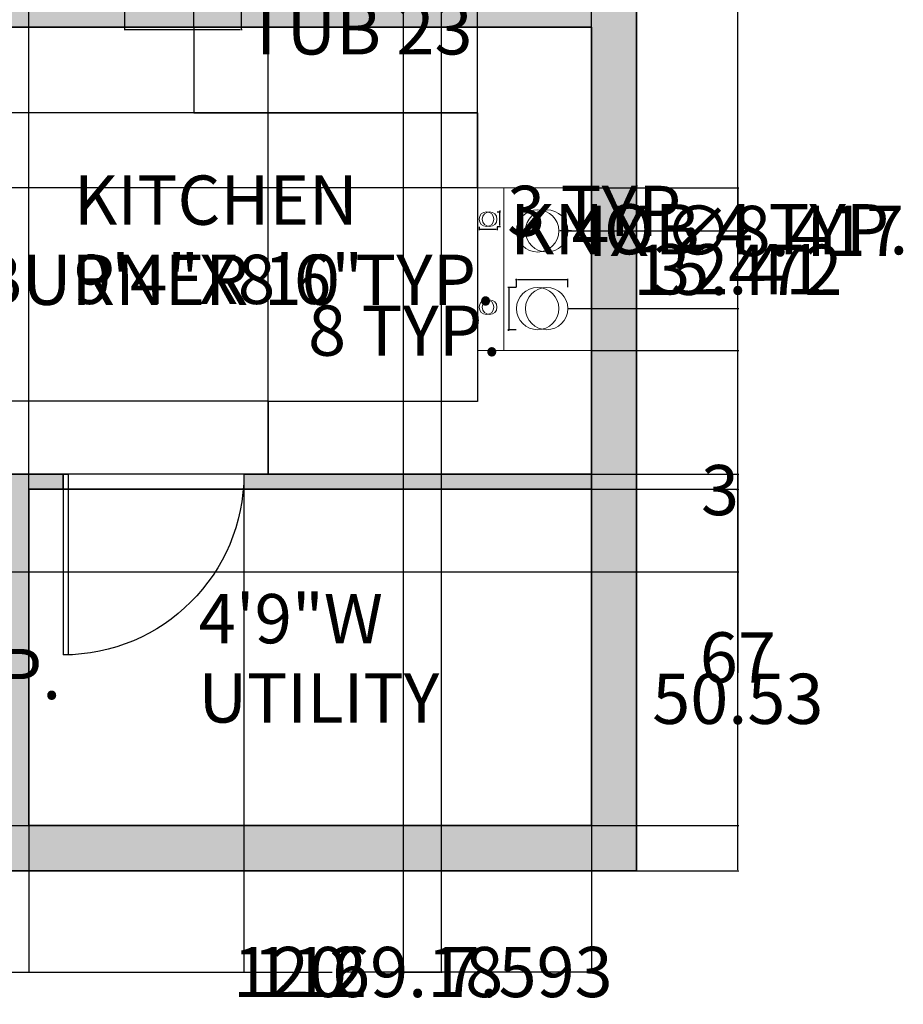
# Model space of a CAD drawing. Units: inches. Extents: x -75 to 484, y -248 to 214.
# Tile 5 of 7: x 291 to 467, y -248 to -52. Entities that reach past the tile are written whole.
import ezdxf

# ---------------------------------------------------------------- set-up
doc = ezdxf.new("R2010")
doc.units = ezdxf.units.IN
doc.header["$MEASUREMENT"] = 0
for name, color, linetype, lineweight in [('A-ANNO-DIMS', 2, 'Continuous', 18), ('A-AREA-IDEN', 7, 'Continuous', 18), ('A-DOOR', 3, 'Continuous', 25), ('A-EQPM', 9, 'Continuous', 18), ('A-FLOR-CASE', 9, 'Continuous', 25), ('A-WALL', 7, 'Continuous', 35)]:
    doc.layers.add(name, color=color, linetype=linetype, lineweight=lineweight)
doc.layers.add('A-WALL-PATT', color=252, linetype='Continuous', lineweight=9, true_color=0x939598)
doc.styles.get("Standard").update_dxf_attribs({"font": 'arial.ttf'})
doc.dimstyles.get("Standard").update_dxf_attribs({"dimtxt": 10, "dimasz": 0.18, "dimexe": 0.18, "dimexo": 0.0625, "dimgap": 0.09, "dimtad": 0, "dimtih": 1, "dimtoh": 1, "dimdec": 0, "dimzin": 0, "dimdsep": 46, "dimlunit": 3, "dimtxsty": 'Standard', "dimcen": 0.09, "dimadec": 0, "dimazin": 0, "dimtfac": 1, "dimtdec": 0, "dimtofl": 0, "dimtmove": 0, "dimatfit": 3, "dimfxl": 1, "dimtolj": 1, "dimtzin": 0, "dimarcsym": 0})

# ---------------------------------------------------------------- blocks, each defined once
blk = doc.blocks.new('DOOR-SINGLE-36')
for p, q in [((35, 36), (35, 0)), ((36, 36), (36, 0))]:
    blk.add_line(p, q)
blk.add_arc((36, 36), 36, 180, 270)
blk = doc.blocks.new('COOKTOP-BURNER')
for centre in [(4.21, 4.21), (6.01, 4.21)]:
    blk.add_circle(centre, 4.21)
blk = doc.blocks.new('COOKTOP-KNOB')
for centre in [(1.47, 1.47), (2.08, 1.47)]:
    blk.add_circle(centre, 1.47)
blk = doc.blocks.new('*D21')
at = {"layer": 'A-ANNO-DIMS', "color": 0, "lineweight": -2, "transparency": 16777216}
for p, q in [((204.49, -180.49), (207.14, -182.4)), ((207, -182.29), (207.1, -182.15)), ((207.1, -182.15), (207.28, -182.15)), ((194.83, -199.19), (206.89, -182.44)), ((192.22, -197.53), (194.87, -199.44))]:
    blk.add_line(p, q, dxfattribs=at)
at = {"layer": 'A-ANNO-DIMS', "color": 0, "transparency": 16777216}
for points in [[(206.87, -182.42), (206.92, -182.46), (207, -182.29)], [(194.8, -199.17), (194.85, -199.2), (194.72, -199.33)]]:
    blk.add_solid(points, dxfattribs=at)
at = {"layer": 'Defpoints', "color": 0, "transparency": 16777216}
for p in [(204.44, -180.45), (207, -182.29), (192.17, -197.49)]:
    blk.add_point(p, dxfattribs=at)
at = {"layer": 'A-ANNO-DIMS', "color": 0, "transparency": 16777216, "insert": (255.32, -182.15), "char_height": 10, "attachment_point": 5}
blk.add_mtext('\\A1;CHAIR 21 TYP.', dxfattribs=at)
blk = doc.blocks.new('*D35')
at = {"layer": 'A-ANNO-DIMS', "color": 0, "lineweight": -2, "transparency": 16777216}
for p, q in [((312.26, -50.35), (312.26, -53.95)), ((335.49, -50.35), (335.49, -53.95)), ((312.44, -53.77), (335.31, -53.77)), ((335.49, -53.77), (335.67, -53.77))]:
    blk.add_line(p, q, dxfattribs=at)
at = {"layer": 'A-ANNO-DIMS', "color": 0, "transparency": 16777216}
for points in [[(312.44, -53.74), (312.44, -53.8), (312.26, -53.77)], [(335.31, -53.74), (335.31, -53.8), (335.49, -53.77)]]:
    blk.add_solid(points, dxfattribs=at)
at = {"layer": 'Defpoints', "color": 0, "transparency": 16777216}
for p in [(312.26, -50.29), (335.49, -50.29), (335.49, -53.77)]:
    blk.add_point(p, dxfattribs=at)
at = {"layer": 'A-ANNO-DIMS', "color": 0, "transparency": 16777216, "insert": (358.96, -53.77), "char_height": 10, "attachment_point": 5}
blk.add_mtext('\\A1;TUB 23', dxfattribs=at)
blk = doc.blocks.new('*D37')
at = {"layer": 'A-ANNO-DIMS', "color": 0, "lineweight": -2, "transparency": 16777216}
for p, q in [((390.31, -103.63), (390.13, -103.63)), ((390.31, -105.1), (390.31, -103.45)), ((400.34, -103.63), (390.49, -103.63)), ((400.52, -105.1), (400.52, -103.45))]:
    blk.add_line(p, q, dxfattribs=at)
at = {"layer": 'A-ANNO-DIMS', "color": 0, "transparency": 16777216}
for points in [[(390.49, -103.6), (390.49, -103.66), (390.31, -103.63)], [(400.34, -103.6), (400.34, -103.66), (400.52, -103.63)]]:
    blk.add_solid(points, dxfattribs=at)
at = {"layer": 'Defpoints', "color": 0, "transparency": 16777216}
for p in [(390.31, -103.63), (390.31, -105.16), (400.52, -105.16)]:
    blk.add_point(p, dxfattribs=at)
at = {"layer": 'A-ANNO-DIMS', "color": 0, "transparency": 16777216, "insert": (334.48, -103.63), "char_height": 10, "attachment_point": 5}
blk.add_mtext('\\A1;BURNER 10 TYP.', dxfattribs=at)
blk = doc.blocks.new('*D38')
at = {"layer": 'A-ANNO-DIMS', "color": 0, "lineweight": -2, "transparency": 16777216}
for p, q in [((390.24, -105.16), (388.59, -105.16)), ((388.77, -105.34), (388.77, -113.4)), ((390.24, -113.58), (388.59, -113.58)), ((388.77, -113.58), (388.77, -113.76)), ((388.77, -113.76), (388.59, -113.76))]:
    blk.add_line(p, q, dxfattribs=at)
at = {"layer": 'A-ANNO-DIMS', "color": 0, "transparency": 16777216}
for points in [[(388.74, -105.34), (388.8, -105.34), (388.77, -105.16)], [(388.74, -113.4), (388.8, -113.4), (388.77, -113.58)]]:
    blk.add_solid(points, dxfattribs=at)
at = {"layer": 'Defpoints', "color": 0, "transparency": 16777216}
for p in [(390.31, -105.16), (388.77, -113.58), (390.31, -113.58)]:
    blk.add_point(p, dxfattribs=at)
at = {"layer": 'A-ANNO-DIMS', "color": 0, "transparency": 16777216, "insert": (368.04, -113.76), "char_height": 10, "attachment_point": 5}
blk.add_mtext('\\A1;8 TYP.', dxfattribs=at)
blk = doc.blocks.new('*D39')
at = {"layer": 'A-ANNO-DIMS', "color": 0, "lineweight": -2, "transparency": 16777216}
for p, q in [((382.86, -93.1), (382.86, -93.75)), ((383.04, -93.57), (386.24, -93.57)), ((386.42, -93.1), (386.42, -93.75)), ((386.42, -93.57), (386.6, -93.57))]:
    blk.add_line(p, q, dxfattribs=at)
at = {"layer": 'A-ANNO-DIMS', "color": 0, "transparency": 16777216}
for points in [[(383.04, -93.54), (383.04, -93.6), (382.86, -93.57)], [(386.24, -93.54), (386.24, -93.6), (386.42, -93.57)]]:
    blk.add_solid(points, dxfattribs=at)
at = {"layer": 'Defpoints', "color": 0, "transparency": 16777216}
for p in [(382.86, -93.04), (386.42, -93.04), (386.42, -93.57)]:
    blk.add_point(p, dxfattribs=at)
at = {"layer": 'A-ANNO-DIMS', "color": 0, "transparency": 16777216, "insert": (428.66, -93.57), "char_height": 10, "attachment_point": 5}
blk.add_mtext('\\A1;KNOB 4 TYP.', dxfattribs=at)
blk = doc.blocks.new('*D40')
at = {"layer": 'A-ANNO-DIMS', "color": 0, "lineweight": -2, "transparency": 16777216}
for p, q in [((386.48, -90.09), (387.13, -90.09)), ((386.95, -90.09), (386.95, -89.91)), ((386.95, -89.91), (387.13, -89.91)), ((386.95, -92.86), (386.95, -90.27)), ((386.48, -93.04), (387.13, -93.04))]:
    blk.add_line(p, q, dxfattribs=at)
at = {"layer": 'A-ANNO-DIMS', "color": 0, "transparency": 16777216}
for points in [[(386.92, -90.27), (386.98, -90.27), (386.95, -90.09)], [(386.92, -92.86), (386.98, -92.86), (386.95, -93.04)]]:
    blk.add_solid(points, dxfattribs=at)
at = {"layer": 'Defpoints', "color": 0, "transparency": 16777216}
for p in [(386.42, -90.09), (386.95, -90.09), (386.42, -93.04)]:
    blk.add_point(p, dxfattribs=at)
at = {"layer": 'A-ANNO-DIMS', "color": 0, "transparency": 16777216, "insert": (407.67, -89.91), "char_height": 10, "attachment_point": 5}
blk.add_mtext('\\A1;3 TYP.', dxfattribs=at)
blk = doc.blocks.new('*D42')
at = {"layer": 'A-ANNO-DIMS', "color": 0, "lineweight": -2, "transparency": 16777216}
for p, q in [((414.27, 147.66), (434.54, 147.66)), ((434.36, 147.48), (434.36, -31.64)), ((434.36, -221.16), (434.36, -42.04)), ((414.27, -221.34), (434.54, -221.34))]:
    blk.add_line(p, q, dxfattribs=at)
at = {"layer": 'A-ANNO-DIMS', "color": 0, "transparency": 16777216}
for points in [[(434.33, 147.48), (434.39, 147.48), (434.36, 147.66)], [(434.33, -221.16), (434.39, -221.16), (434.36, -221.34)]]:
    blk.add_solid(points, dxfattribs=at)
at = {"layer": 'Defpoints', "color": 0, "transparency": 16777216}
for p in [(414.21, 147.66), (414.21, -221.34), (434.36, -221.34)]:
    blk.add_point(p, dxfattribs=at)
at = {"layer": 'A-ANNO-DIMS', "color": 0, "transparency": 16777216, "insert": (434.36, -36.84), "char_height": 10, "attachment_point": 5}
blk.add_mtext('\\A1;369', dxfattribs=at)
blk = doc.blocks.new('*D55')
at = {"layer": 'A-ANNO-DIMS', "color": 0, "lineweight": -2, "transparency": 16777216}
for p, q in [((293.21, -212.41), (293.21, -241.67)), ((405.21, -212.41), (405.21, -241.67)), ((293.39, -241.49), (338.59, -241.49)), ((405.03, -241.49), (359.82, -241.49))]:
    blk.add_line(p, q, dxfattribs=at)
at = {"layer": 'A-ANNO-DIMS', "color": 0, "transparency": 16777216}
for points in [[(293.39, -241.46), (293.39, -241.52), (293.21, -241.49)], [(405.03, -241.46), (405.03, -241.52), (405.21, -241.49)]]:
    blk.add_solid(points, dxfattribs=at)
at = {"layer": 'Defpoints', "color": 0, "transparency": 16777216}
for p in [(293.21, -212.34), (405.21, -212.34), (405.21, -241.49)]:
    blk.add_point(p, dxfattribs=at)
at = {"layer": 'A-ANNO-DIMS', "color": 0, "transparency": 16777216, "insert": (349.21, -241.49), "char_height": 10, "attachment_point": 5}
blk.add_mtext('\\A1;112', dxfattribs=at)
blk = doc.blocks.new('*D57')
at = {"layer": 'A-ANNO-DIMS', "color": 0, "lineweight": -2, "transparency": 16777216}
for p, q in [((285.21, -212.28), (285.21, 167.99)), ((285.39, 167.81), (285.82, 167.81)), ((293.03, 167.81), (292.59, 167.81)), ((293.21, -212.28), (293.21, 167.99))]:
    blk.add_line(p, q, dxfattribs=at)
at = {"layer": 'A-ANNO-DIMS', "color": 0, "transparency": 16777216}
for points in [[(285.39, 167.84), (285.39, 167.78), (285.21, 167.81)], [(293.03, 167.84), (293.03, 167.78), (293.21, 167.81)]]:
    blk.add_solid(points, dxfattribs=at)
at = {"layer": 'Defpoints', "color": 0, "transparency": 16777216}
for p in [(285.21, 167.81), (285.21, -212.34), (293.21, -212.34)]:
    blk.add_point(p, dxfattribs=at)
at = {"layer": 'A-ANNO-DIMS', "color": 0, "transparency": 16777216, "insert": (289.21, 167.81), "char_height": 10, "attachment_point": 5}
blk.add_mtext('\\A1;8', dxfattribs=at)
blk = doc.blocks.new('*D62')
at = {"layer": 'A-ANNO-DIMS', "color": 0, "lineweight": -2, "transparency": 16777216}
for p, q in [((336.03, -142.41), (336.03, -241.67)), ((405.21, -145.41), (405.21, -241.67)), ((336.21, -241.49), (353.62, -241.49)), ((405.03, -241.49), (387.62, -241.49))]:
    blk.add_line(p, q, dxfattribs=at)
at = {"layer": 'A-ANNO-DIMS', "color": 0, "transparency": 16777216}
for points in [[(336.21, -241.46), (336.21, -241.52), (336.03, -241.49)], [(405.03, -241.46), (405.03, -241.52), (405.21, -241.49)]]:
    blk.add_solid(points, dxfattribs=at)
at = {"layer": 'Defpoints', "color": 0, "transparency": 16777216}
for p in [(336.03, -142.34), (405.21, -145.34), (405.21, -241.49)]:
    blk.add_point(p, dxfattribs=at)
at = {"layer": 'A-ANNO-DIMS', "color": 0, "transparency": 16777216, "insert": (370.62, -241.49), "char_height": 10, "attachment_point": 5}
blk.add_mtext('\\A1;69.18', dxfattribs=at)
blk = doc.blocks.new('*D63')
at = {"layer": 'A-ANNO-DIMS', "color": 0, "lineweight": -2, "transparency": 16777216}
for p, q in [((405.27, -145.34), (434.54, -145.34)), ((434.36, -145.52), (434.36, -173.65)), ((434.36, -212.16), (434.36, -184.04)), ((405.27, -212.34), (434.54, -212.34))]:
    blk.add_line(p, q, dxfattribs=at)
at = {"layer": 'A-ANNO-DIMS', "color": 0, "transparency": 16777216}
for points in [[(434.33, -145.52), (434.39, -145.52), (434.36, -145.34)], [(434.33, -212.16), (434.39, -212.16), (434.36, -212.34)]]:
    blk.add_solid(points, dxfattribs=at)
at = {"layer": 'Defpoints', "color": 0, "transparency": 16777216}
for p in [(405.21, -145.34), (405.21, -212.34), (434.36, -212.34)]:
    blk.add_point(p, dxfattribs=at)
at = {"layer": 'A-ANNO-DIMS', "color": 0, "transparency": 16777216, "insert": (434.36, -178.84), "char_height": 10, "attachment_point": 5}
blk.add_mtext('\\A1;67', dxfattribs=at)
blk = doc.blocks.new('*D64')
at = {"layer": 'A-ANNO-DIMS', "color": 0, "lineweight": -2, "transparency": 16777216}
for p, q in [((326.06, -53.28), (326.06, 167.99)), ((326.24, 167.81), (348.67, 167.81)), ((405.03, 167.81), (382.59, 167.81)), ((405.21, -53.28), (405.21, 167.99))]:
    blk.add_line(p, q, dxfattribs=at)
at = {"layer": 'A-ANNO-DIMS', "color": 0, "transparency": 16777216}
for points in [[(326.24, 167.84), (326.24, 167.78), (326.06, 167.81)], [(405.03, 167.84), (405.03, 167.78), (405.21, 167.81)]]:
    blk.add_solid(points, dxfattribs=at)
at = {"layer": 'Defpoints', "color": 0, "transparency": 16777216}
for p in [(405.21, 167.81), (326.06, -53.34), (405.21, -53.34)]:
    blk.add_point(p, dxfattribs=at)
at = {"layer": 'A-ANNO-DIMS', "color": 0, "transparency": 16777216, "insert": (365.63, 167.81), "char_height": 10, "attachment_point": 5}
blk.add_mtext('\\A1;79.15', dxfattribs=at)
blk = doc.blocks.new('*D65')
at = {"layer": 'A-ANNO-DIMS', "color": 0, "lineweight": -2, "transparency": 16777216}
for p, q in [((340.87, -142.28), (340.87, 167.99)), ((341.05, 167.81), (356.07, 167.81)), ((405.03, 167.81), (390.01, 167.81)), ((405.21, -142.28), (405.21, 167.99))]:
    blk.add_line(p, q, dxfattribs=at)
at = {"layer": 'A-ANNO-DIMS', "color": 0, "transparency": 16777216}
for points in [[(341.05, 167.84), (341.05, 167.78), (340.87, 167.81)], [(405.03, 167.84), (405.03, 167.78), (405.21, 167.81)]]:
    blk.add_solid(points, dxfattribs=at)
at = {"layer": 'Defpoints', "color": 0, "transparency": 16777216}
for p in [(405.21, 167.81), (340.87, -142.34), (405.21, -142.34)]:
    blk.add_point(p, dxfattribs=at)
at = {"layer": 'A-ANNO-DIMS', "color": 0, "transparency": 16777216, "insert": (373.04, 167.81), "char_height": 10, "attachment_point": 5}
blk.add_mtext('\\A1;64.34', dxfattribs=at)
blk = doc.blocks.new('*D66')
at = {"layer": 'A-ANNO-DIMS', "color": 0, "lineweight": -2, "transparency": 16777216}
for p, q in [((382.57, -85.27), (382.57, 167.99)), ((382.75, 167.81), (405.03, 167.81)), ((405.21, -85.27), (405.21, 167.99)), ((405.21, 167.81), (405.39, 167.81))]:
    blk.add_line(p, q, dxfattribs=at)
at = {"layer": 'A-ANNO-DIMS', "color": 0, "transparency": 16777216}
for points in [[(382.75, 167.84), (382.75, 167.78), (382.57, 167.81)], [(405.03, 167.84), (405.03, 167.78), (405.21, 167.81)]]:
    blk.add_solid(points, dxfattribs=at)
at = {"layer": 'Defpoints', "color": 0, "transparency": 16777216}
for p in [(405.21, 167.81), (382.57, -85.33), (405.21, -85.33)]:
    blk.add_point(p, dxfattribs=at)
at = {"layer": 'A-ANNO-DIMS', "color": 0, "transparency": 16777216, "insert": (426.32, 167.81), "char_height": 10, "attachment_point": 5}
blk.add_mtext('\\A1;22.643', dxfattribs=at)
blk = doc.blocks.new('*D67')
at = {"layer": 'A-ANNO-DIMS', "color": 0, "lineweight": -2, "transparency": 16777216}
for p, q in [((325.99, -53.34), (-5.12, -53.34)), ((-4.94, -53.52), (-4.94, -56.68)), ((-4.94, -70.23), (-4.94, -67.07)), ((325.99, -70.41), (-5.12, -70.41))]:
    blk.add_line(p, q, dxfattribs=at)
at = {"layer": 'A-ANNO-DIMS', "color": 0, "transparency": 16777216}
for points in [[(-4.97, -53.52), (-4.91, -53.52), (-4.94, -53.34)], [(-4.97, -70.23), (-4.91, -70.23), (-4.94, -70.41)]]:
    blk.add_solid(points, dxfattribs=at)
at = {"layer": 'Defpoints', "color": 0, "transparency": 16777216}
for p in [(326.06, -53.34), (-4.94, -70.41), (326.06, -70.41)]:
    blk.add_point(p, dxfattribs=at)
at = {"layer": 'A-ANNO-DIMS', "color": 0, "transparency": 16777216, "insert": (-4.94, -61.88), "char_height": 10, "attachment_point": 5}
blk.add_mtext('\\A1;17.068', dxfattribs=at)
blk = doc.blocks.new('*D68')
at = {"layer": 'A-ANNO-DIMS', "color": 0, "lineweight": -2, "transparency": 16777216}
for p, q in [((340.8, -127.84), (-5.12, -127.84)), ((-4.94, -128.02), (-4.94, -129.9)), ((-4.94, -142.16), (-4.94, -140.29)), ((340.8, -142.34), (-5.12, -142.34))]:
    blk.add_line(p, q, dxfattribs=at)
at = {"layer": 'A-ANNO-DIMS', "color": 0, "transparency": 16777216}
for points in [[(-4.97, -128.02), (-4.91, -128.02), (-4.94, -127.84)], [(-4.97, -142.16), (-4.91, -142.16), (-4.94, -142.34)]]:
    blk.add_solid(points, dxfattribs=at)
at = {"layer": 'Defpoints', "color": 0, "transparency": 16777216}
for p in [(340.87, -127.84), (-4.94, -142.34), (340.87, -142.34)]:
    blk.add_point(p, dxfattribs=at)
at = {"layer": 'A-ANNO-DIMS', "color": 0, "transparency": 16777216, "insert": (-4.94, -135.09), "char_height": 10, "attachment_point": 5}
blk.add_mtext('\\A1;14.5', dxfattribs=at)
blk = doc.blocks.new('*D70')
at = {"layer": 'A-ANNO-DIMS', "color": 0, "lineweight": -2, "transparency": 16777216}
for p, q in [((285.21, -53.41), (285.21, -241.67)), ((405.21, -53.41), (405.21, -241.67)), ((285.39, -241.49), (334.56, -241.49)), ((405.03, -241.49), (355.86, -241.49))]:
    blk.add_line(p, q, dxfattribs=at)
at = {"layer": 'A-ANNO-DIMS', "color": 0, "transparency": 16777216}
for points in [[(285.39, -241.46), (285.39, -241.52), (285.21, -241.49)], [(405.03, -241.46), (405.03, -241.52), (405.21, -241.49)]]:
    blk.add_solid(points, dxfattribs=at)
at = {"layer": 'Defpoints', "color": 0, "transparency": 16777216}
for p in [(285.21, -53.34), (405.21, -53.34), (405.21, -241.49)]:
    blk.add_point(p, dxfattribs=at)
at = {"layer": 'A-ANNO-DIMS', "color": 0, "transparency": 16777216, "insert": (345.21, -241.49), "char_height": 10, "attachment_point": 5}
blk.add_mtext('\\A1;120', dxfattribs=at)
blk = doc.blocks.new('*D71')
at = {"layer": 'A-ANNO-DIMS', "color": 0, "lineweight": -2, "transparency": 16777216}
for p, q in [((405.27, -85.33), (434.54, -85.33)), ((434.36, -85.51), (434.36, -96.34)), ((434.36, -117.56), (434.36, -106.74)), ((405.27, -117.74), (434.54, -117.74))]:
    blk.add_line(p, q, dxfattribs=at)
at = {"layer": 'A-ANNO-DIMS', "color": 0, "transparency": 16777216}
for points in [[(434.33, -85.51), (434.39, -85.51), (434.36, -85.33)], [(434.33, -117.56), (434.39, -117.56), (434.36, -117.74)]]:
    blk.add_solid(points, dxfattribs=at)
at = {"layer": 'Defpoints', "color": 0, "transparency": 16777216}
for p in [(405.21, -85.33), (405.21, -117.74), (434.36, -117.74)]:
    blk.add_point(p, dxfattribs=at)
at = {"layer": 'A-ANNO-DIMS', "color": 0, "transparency": 16777216, "insert": (434.36, -101.54), "char_height": 10, "attachment_point": 5}
blk.add_mtext('\\A1;32.41', dxfattribs=at)
blk = doc.blocks.new('*D72')
at = {"layer": 'A-ANNO-DIMS', "color": 0, "lineweight": -2, "transparency": 16777216}
for p, q in [((382.5, -70.41), (-5.12, -70.41)), ((-4.94, -70.59), (-4.94, -72.68)), ((-4.94, -85.15), (-4.94, -83.07)), ((382.5, -85.33), (-5.12, -85.33))]:
    blk.add_line(p, q, dxfattribs=at)
at = {"layer": 'A-ANNO-DIMS', "color": 0, "transparency": 16777216}
for points in [[(-4.97, -70.59), (-4.91, -70.59), (-4.94, -70.41)], [(-4.97, -85.15), (-4.91, -85.15), (-4.94, -85.33)]]:
    blk.add_solid(points, dxfattribs=at)
at = {"layer": 'Defpoints', "color": 0, "transparency": 16777216}
for p in [(382.57, -70.41), (-4.94, -85.33), (382.57, -85.33)]:
    blk.add_point(p, dxfattribs=at)
at = {"layer": 'A-ANNO-DIMS', "color": 0, "transparency": 16777216, "insert": (-4.94, -77.87), "char_height": 10, "attachment_point": 5}
blk.add_mtext('\\A1;14.92', dxfattribs=at)
blk = doc.blocks.new('*D73')
at = {"layer": 'A-ANNO-DIMS', "color": 0, "lineweight": -2, "transparency": 16777216}
for p, q in [((405.27, -142.34), (434.54, -142.34)), ((434.36, -142.52), (434.36, -145.16)), ((405.27, -145.34), (434.54, -145.34)), ((434.36, -145.52), (434.18, -145.52)), ((434.36, -145.34), (434.36, -145.52))]:
    blk.add_line(p, q, dxfattribs=at)
at = {"layer": 'A-ANNO-DIMS', "color": 0, "transparency": 16777216}
for points in [[(434.33, -142.52), (434.39, -142.52), (434.36, -142.34)], [(434.33, -145.16), (434.39, -145.16), (434.36, -145.34)]]:
    blk.add_solid(points, dxfattribs=at)
at = {"layer": 'Defpoints', "color": 0, "transparency": 16777216}
for p in [(405.21, -142.34), (405.21, -145.34), (434.36, -145.34)]:
    blk.add_point(p, dxfattribs=at)
at = {"layer": 'A-ANNO-DIMS', "color": 0, "transparency": 16777216, "insert": (430.82, -145.52), "char_height": 10, "attachment_point": 5}
blk.add_mtext('\\A1;3', dxfattribs=at)
blk = doc.blocks.new('*D74')
at = {"layer": 'A-ANNO-DIMS', "color": 0, "lineweight": -2, "transparency": 16777216}
for p, q in [((24.27, -161.82), (434.54, -161.82)), ((434.36, -162), (434.36, -181.88)), ((434.36, -212.16), (434.36, -192.28)), ((24.27, -212.34), (434.54, -212.34))]:
    blk.add_line(p, q, dxfattribs=at)
at = {"layer": 'A-ANNO-DIMS', "color": 0, "transparency": 16777216}
for points in [[(434.33, -162), (434.39, -162), (434.36, -161.82)], [(434.33, -212.16), (434.39, -212.16), (434.36, -212.34)]]:
    blk.add_solid(points, dxfattribs=at)
at = {"layer": 'Defpoints', "color": 0, "transparency": 16777216}
for p in [(24.21, -161.82), (434.36, -161.82), (24.21, -212.34)]:
    blk.add_point(p, dxfattribs=at)
at = {"layer": 'A-ANNO-DIMS', "color": 0, "transparency": 16777216, "insert": (434.36, -187.08), "char_height": 10, "attachment_point": 5}
blk.add_mtext('\\A1;50.53', dxfattribs=at)
blk = doc.blocks.new('*D80')
at = {"layer": 'A-ANNO-DIMS', "color": 0, "lineweight": -2, "transparency": 16777216}
for p, q in [((367.71, -42.41), (367.71, -241.67)), ((375.3, -50.41), (375.3, -241.67)), ((367.89, -241.49), (375.12, -241.49)), ((375.3, -241.49), (375.48, -241.49))]:
    blk.add_line(p, q, dxfattribs=at)
at = {"layer": 'A-ANNO-DIMS', "color": 0, "transparency": 16777216}
for points in [[(367.89, -241.46), (367.89, -241.52), (367.71, -241.49)], [(375.12, -241.46), (375.12, -241.52), (375.3, -241.49)]]:
    blk.add_solid(points, dxfattribs=at)
at = {"layer": 'Defpoints', "color": 0, "transparency": 16777216}
for p in [(367.71, -42.34), (375.3, -50.34), (375.3, -241.49)]:
    blk.add_point(p, dxfattribs=at)
at = {"layer": 'A-ANNO-DIMS', "color": 0, "transparency": 16777216, "insert": (392.4, -241.49), "char_height": 10, "attachment_point": 5}
blk.add_mtext('\\A1;7.593', dxfattribs=at)
blk = doc.blocks.new('*D82')
at = {"layer": 'A-ANNO-DIMS', "color": 0, "lineweight": -2, "transparency": 16777216}
for p, q in [((400.59, -93.9), (434.54, -93.9)), ((434.36, -94.08), (434.36, -96.44)), ((434.36, -109.19), (434.36, -106.83)), ((400.59, -109.37), (434.54, -109.37))]:
    blk.add_line(p, q, dxfattribs=at)
at = {"layer": 'A-ANNO-DIMS', "color": 0, "transparency": 16777216}
for points in [[(434.33, -94.08), (434.39, -94.08), (434.36, -93.9)], [(434.33, -109.19), (434.39, -109.19), (434.36, -109.37)]]:
    blk.add_solid(points, dxfattribs=at)
at = {"layer": 'Defpoints', "color": 0, "transparency": 16777216}
for p in [(400.52, -93.9), (400.52, -109.37), (434.36, -109.37)]:
    blk.add_point(p, dxfattribs=at)
at = {"layer": 'A-ANNO-DIMS', "color": 0, "transparency": 16777216, "insert": (434.36, -101.64), "char_height": 10, "attachment_point": 5}
blk.add_mtext('\\A1;15.472', dxfattribs=at)
blk = doc.blocks.new('*D88')
at = {"layer": 'A-ANNO-DIMS', "color": 0, "lineweight": -2, "transparency": 16777216}
for p, q in [((394.42, -93.9), (394.6, -93.9)), ((394.51, -93.99), (394.51, -93.81)), ((401.25, -93.9), (398.9, -93.9))]:
    blk.add_line(p, q, dxfattribs=at)
at = {"layer": 'A-ANNO-DIMS', "color": 0, "transparency": 16777216}
blk.add_solid([(398.9, -93.87), (398.9, -93.93), (398.72, -93.9)], dxfattribs=at)
at = {"layer": 'Defpoints', "color": 0, "transparency": 16777216}
for p in [(390.31, -93.9), (398.72, -93.9)]:
    blk.add_point(p, dxfattribs=at)
at = {"layer": 'A-ANNO-DIMS', "color": 0, "transparency": 16777216, "insert": (434.33, -93.9), "char_height": 10, "attachment_point": 5}
blk.add_mtext('\\A1;4X ∅8.417', dxfattribs=at)

msp = doc.modelspace()

# ---------------------------------------------------------------- hatches: boundary and pattern name
at = {"layer": 'A-WALL-PATT'}
h = msp.add_hatch(color=256, dxfattribs=at)
h.dxf.hatch_style = 1
h.paths.add_polyline_path([(184.9004, 147.6567), (15.2094, 147.6567), (15.2094, 92.5031), (24.2094, 92.5031), (24.2094, 138.6567), (186.0436, 138.6567, -0.06325422)])
h.paths.add_polyline_path([(414.2094, 147.6567), (249.2094, 147.6567), (220.9004, 147.6567), (220.9004, 138.6567), (240.2094, 138.6567), (240.2094, 18.6567), (240.2094, 9.6567), (249.2094, 9.6567), (249.2094, 45.6567), (249.2094, 138.6567), (405.2094, 138.6567), (405.2094, 98.3029), (414.2094, 98.3029)])
h.paths.add_polyline_path([(159.2094, 18.6567), (24.2094, 18.6567), (24.2094, 44.5861), (15.2094, 44.5861), (15.2094, 9.6567), (15.2094, -3.1791), (24.2094, -3.1791), (24.2094, 9.6567), (132.2094, 9.6567), (132.2094, -50.3433), (83.7394, -50.3433), (83.7394, -53.3433), (132.2094, -53.3433), (159.2094, -53.3433), (159.2094, -50.3433), (135.2094, -50.3433), (135.2094, 9.6567), (159.2094, 9.6567)])
h.paths.add_polyline_path([(53.8898, -50.3433), (24.2094, -50.3433), (24.2094, -27.303), (15.2094, -27.303), (15.2094, -50.3433), (15.2094, -53.3433), (15.2094, -74.0487), (24.2094, -74.0487), (24.2094, -53.3433), (53.7394, -53.3433, -0.02504709)])
h.paths.add_polyline_path([(24.2094, -121.9657), (15.2094, -121.9657), (15.2094, -212.3433), (15.2094, -221.3433), (24.2094, -221.3433), (84.3017, -221.3433), (84.3017, -212.3433), (24.2094, -212.3433)])
h.paths.add_polyline_path([(414.2094, -155.3433), (414.2094, -53.3433), (414.2094, -50.3433), (414.2094, -36.8417), (405.2094, -36.8417), (405.2094, -50.3433), (309.2094, -50.3433), (309.2094, 16.0463), (324.2573, 16.0463), (324.2573, 18.6567), (284.0663, 18.6567, -0.06325422), (285.2094, 9.6567), (306.2094, 9.6567), (306.2094, -50.3433), (285.2094, -50.3433), (285.2094, -53.3433), (309.2094, -53.3433), (405.2094, -53.3433), (405.2094, -212.3433), (293.2094, -212.3433), (293.2094, -158.3433), (293.2094, -145.3433), (300.0339, -145.3433), (300.0339, -142.3433), (285.2094, -142.3433), (159.2094, -142.3433), (159.2094, -89.3433, -0.02086055), (156.2094, -89.218), (156.2094, -212.3433), (131.9001, -212.3433), (131.9001, -221.3433), (156.2094, -221.3433), (165.2094, -221.3433), (285.2094, -221.3433), (288.6713, -221.3433), (293.2094, -221.3433), (405.2094, -221.3433), (414.2094, -221.3433)])
h.paths.add_polyline_path([(165.2094, -212.3433), (165.2094, -151.3433), (285.2094, -151.3433), (285.2094, -212.3433)], flags=16)
h.paths.add_polyline_path([(189.462, -195.5437), (182.159, -190.2838, -0.23606798), (182.5164, -188.0765), (181.7049, -187.4921), (185.5037, -182.2177), (184.648, -181.6013, -0.04492589), (180.0821, -186.3232), (179.2706, -185.7388), (189.206, -171.9443), (190.0174, -172.5287, -0.04492589), (186.9857, -178.3556), (187.8415, -178.9719), (191.6403, -173.6976), (192.4517, -174.282, -0.23606798), (194.432, -173.2435), (201.735, -178.5034, -0.23606798), (201.3776, -180.7107), (202.189, -181.2952, -0.11764706), (192.2537, -195.0897), (191.4423, -194.5053, -0.23606798)], flags=0)
h.paths.add_polyline_path([(253.751, -177.9543), (254.5293, -177.3263, -0.23606798), (254.0517, -175.1419), (261.056, -169.4904, -0.23606798), (263.0902, -170.419), (263.8684, -169.7911), (267.95, -174.8498), (268.7708, -174.1875, -0.04492589), (265.425, -168.5352), (266.2032, -167.9073), (276.8782, -181.1378), (276.0999, -181.7657, -0.04492589), (271.2826, -177.3006), (270.4618, -177.9629), (274.5434, -183.0216), (273.7651, -183.6495, -0.23606798), (274.2427, -185.834), (267.2383, -191.4854, -0.23606798), (265.2042, -190.5568), (264.4259, -191.1848, -0.11764706)], flags=0)
h.paths.add_polyline_path([(405.2094, -142.3433), (336.0339, -142.3433, -0.02086055), (335.9087, -145.3433), (405.2094, -145.3433)], flags=17)
h.paths.add_polyline_path([(414.2094, 50.4831), (405.2094, 50.4831), (405.2094, 18.6567), (354.2573, 18.6567, -0.02178446), (354.1435, 16.0463), (405.2094, 16.0463), (405.2094, -14.6494), (414.2094, -14.6494), (414.2094, 9.6567)])
h.paths.add_polyline_path([(200.2091, -179.9247), (255.2702, -179.9247), (255.2702, -168.0448), (200.2091, -168.0448)], flags=8)
h.paths.add_polyline_path([(200.2352, -167.6036), (249.7883, -167.6036), (249.7883, -155.8804), (200.2352, -155.8804)], flags=8)

# ---------------------------------------------------------------- linework, layer by layer
at = {"layer": 'A-DOOR'}
msp.add_line((300.0339, -142.3433), (301.0339, -142.3433), dxfattribs=at)
at = {"layer": 'A-EQPM'}
msp.add_line((387.7545, -85.3314), (387.7545, -117.7421), dxfattribs=at)
msp.add_lwpolyline([(382.5668, -85.3314), (405.2094, -85.3314), (405.2094, -117.7421), (382.5668, -117.7421)], close=True, dxfattribs=at)
at = {"layer": 'A-FLOR-CASE'}
for p, q in [((326.0553, -53.3433), (326.0553, -70.4114)), ((326.0553, -70.4114), (382.5668, -70.4114)), ((382.5668, -70.4114), (382.5668, -127.8437)), ((382.5668, -127.8437), (340.8661, -127.8437)), ((340.8661, -127.8437), (340.8661, -142.3433))]:
    msp.add_line(p, q, dxfattribs=at)
at = {"layer": 'A-WALL'}
for p, q in [((414.2094, -50.3433), (414.2094, -53.3433)), ((309.2094, -53.3433), (285.2094, -53.3433)), ((405.2094, -53.3433), (309.2094, -53.3433)), ((405.2094, -53.3433), (405.2094, -212.3433)), ((414.2094, -53.3433), (414.2094, -155.3433)), ((301.0339, -142.3433), (285.2094, -142.3433)), ((300.0339, -142.3433), (300.0339, -145.3433)), ((405.2094, -142.3433), (336.0339, -142.3433)), ((293.2094, -212.3433), (293.2094, -145.3433)), ((405.2094, -145.3433), (293.2094, -145.3433)), ((414.2094, -155.3433), (414.2094, -221.3433)), ((293.2094, -212.3433), (293.2094, -158.3433)), ((405.2094, -158.3433), (405.2094, -212.3433)), ((414.2094, -158.3433), (414.2094, -212.3433)), ((405.2094, -212.3433), (293.2094, -212.3433)), ((293.2094, -221.3433), (288.6713, -221.3433)), ((405.2094, -221.3433), (293.2094, -221.3433)), ((414.2094, -221.3433), (405.2094, -221.3433))]:
    msp.add_line(p, q, dxfattribs=at)

# ---------------------------------------------------------------- block references
at = {"layer": 'A-DOOR', "extrusion": (0, 0, -1), "zscale": -1}
msp.add_blockref('DOOR-SINGLE-36', (-336.0339, -178.3433), dxfattribs=at)
at = {"layer": 'A-EQPM'}
for name, p in [('COOKTOP-KNOB', (382.8637, -93.0412)), ('COOKTOP-BURNER', (390.3065, -98.1074)), ('COOKTOP-KNOB', (382.8637, -110.5561))]:
    msp.add_blockref(name, p, dxfattribs=at)
at = {"layer": 'A-EQPM', "rotation": 180}
msp.add_blockref('COOKTOP-BURNER', (400.5232, -105.1627), dxfattribs=at)

# ---------------------------------------------------------------- texts
at = {"layer": 'A-AREA-IDEN'}
for s, p in [('KITCHEN', (302.1992, -92.6869)), ('9\'4"X8\'6"', (302.1992, -108.4628)), ('4\'9"W', (326.9984, -176.032)), ('UTILITY', (326.9984, -191.8079))]:
    msp.add_text(s, height=9.82058, dxfattribs=at).set_placement(p)

# ---------------------------------------------------------------- dimensions: what is measured, and where the dimension line sits
at = {"layer": 'A-ANNO-DIMS'}
for base, p1, p2, override, picture, middle in [((285.2094, 167.8067), (293.2094, -212.3433), (285.2094, -212.3433), {"dimdec": 0, "dimlfac": 1, "dimrnd": 0, "dimzin": 0, "dimdsep": 46, "dimlunit": 2}, '*D57', (289.2094, 167.8067)), ((405.2094, 167.8067), (326.0553, -53.3433), (405.2094, -53.3433), {"dimdec": 2, "dimlfac": 1, "dimrnd": 0, "dimzin": 0, "dimdsep": 46, "dimlunit": 2}, '*D64', (365.6324, 167.8067)), ((405.2094, 167.8067), (340.8661, -142.3433), (405.2094, -142.3433), {"dimdec": 2, "dimlfac": 1, "dimrnd": 0, "dimzin": 0, "dimdsep": 46, "dimlunit": 2}, '*D65', (373.0378, 167.8067)), ((405.2094, 167.8067), (382.5668, -85.3314), (405.2094, -85.3314), {"dimdec": 3, "dimlfac": 1, "dimrnd": 0, "dimzin": 0, "dimdsep": 46, "dimlunit": 2}, '*D66', (426.3218, 167.8067)), ((375.3026, -241.4933), (367.7094, -42.3433), (375.3026, -50.3433), {"dimdec": 3, "dimlfac": 1, "dimrnd": 0, "dimzin": 0, "dimdsep": 46, "dimlunit": 2}, '*D80', (392.4041, -241.4933)), ((405.2094, -241.4933), (285.2094, -53.3433), (405.2094, -53.3433), {"dimdec": 0, "dimlfac": 1, "dimrnd": 0, "dimzin": 0, "dimdsep": 46, "dimlunit": 2}, '*D70', (345.2094, -241.4933)), ((405.2094, -241.4933), (336.0339, -142.3433), (405.2094, -145.3433), {"dimdec": 2, "dimlfac": 1, "dimrnd": 0, "dimzin": 0, "dimdsep": 46, "dimlunit": 2}, '*D62', (370.6216, -241.4933)), ((405.2094, -241.4933), (293.2094, -212.3433), (405.2094, -212.3433), {"dimdec": 0, "dimlfac": 1, "dimrnd": 0, "dimzin": 0, "dimdsep": 46, "dimlunit": 2}, '*D55', (349.2094, -241.4933))]:
    dim = msp.add_linear_dim(base=base, p1=p1, p2=p2, dimstyle='Standard', override=override, dxfattribs=at)
    dim.commit()
    dim.dimension.update_dxf_attribs({"geometry": picture, "text_midpoint": middle})
for base, p1, p2, override, picture, middle in [((434.3594, -221.3433), (414.2094, 147.6567), (414.2094, -221.3433), {"dimdec": 0, "dimlfac": 1, "dimrnd": 0, "dimzin": 0, "dimdsep": 46, "dimlunit": 2}, '*D42', (434.3594, -36.8433)), ((-4.9406, -70.4114), (326.0553, -53.3433), (326.0553, -70.4114), {"dimdec": 3, "dimlfac": 1, "dimrnd": 0, "dimzin": 0, "dimdsep": 46, "dimlunit": 2}, '*D67', (-4.9406, -61.8773)), ((-4.9406, -85.3314), (382.5668, -70.4114), (382.5668, -85.3314), {"dimdec": 2, "dimlfac": 1, "dimrnd": 0, "dimzin": 0, "dimdsep": 46, "dimlunit": 2}, '*D72', (-4.9406, -77.8714)), ((434.3594, -117.7421), (405.2094, -85.3314), (405.2094, -117.7421), {"dimdec": 2, "dimlfac": 1, "dimrnd": 0, "dimzin": 0, "dimdsep": 46, "dimlunit": 2}, '*D71', (434.3594, -101.5367)), ((434.3594, -109.3712), (400.5232, -93.899), (400.5232, -109.3712), {"dimdec": 3, "dimlfac": 1, "dimrnd": 0, "dimzin": 0, "dimdsep": 46, "dimlunit": 2}, '*D82', (434.3594, -101.6351)), ((-4.9406, -142.3433), (340.8661, -127.8437), (340.8661, -142.3433), {"dimdec": 1, "dimlfac": 1, "dimrnd": 0, "dimzin": 0, "dimdsep": 46, "dimlunit": 2}, '*D68', (-4.9406, -135.0935)), ((434.3594, -145.3433), (405.2094, -142.3433), (405.2094, -145.3433), {"dimdec": 0, "dimlfac": 1, "dimrnd": 0, "dimzin": 0, "dimdsep": 46, "dimlunit": 2}, '*D73', (430.8152, -145.5233)), ((434.3594, -212.3433), (405.2094, -145.3433), (405.2094, -212.3433), {"dimdec": 0, "dimlfac": 1, "dimrnd": 0, "dimzin": 0, "dimdsep": 46, "dimlunit": 2}, '*D63', (434.3594, -178.8433)), ((434.3594, -161.8152), (24.2094, -212.3433), (24.2094, -161.8152), {"dimdec": 2, "dimlfac": 1, "dimrnd": 0, "dimzin": 0, "dimdsep": 46, "dimlunit": 2}, '*D74', (434.3594, -187.0792))]:
    dim = msp.add_linear_dim(base=base, p1=p1, p2=p2, angle=90, dimstyle='Standard', override=override, dxfattribs=at)
    dim.commit()
    dim.dimension.update_dxf_attribs({"geometry": picture, "text_midpoint": middle})
for base, p1, p2, text, picture, middle in [((335.4865, -53.773), (312.2619, -50.2893), (335.4865, -50.2893), 'TUB <>', '*D35', (358.9557, -53.773)), ((386.4174, -93.5743), (382.8637, -93.0412), (386.4174, -93.0412), 'KNOB <> TYP.', '*D39', (428.6553, -93.5743))]:
    dim = msp.add_linear_dim(base=base, p1=p1, p2=p2, text=text, dimstyle='Standard', override={"dimdec": 0, "dimlfac": 1, "dimrnd": 0, "dimzin": 0, "dimdsep": 46, "dimlunit": 2}, dxfattribs=at)
    dim.commit()
    dim.dimension.update_dxf_attribs({"geometry": picture, "text_midpoint": middle})
for base, p1, p2, angle, text, picture, middle in [((386.9505, -90.0912), (386.4174, -93.0412), (386.4174, -90.0912), 90, '<> TYP.', '*D40', (407.6707, -89.9112)), ((390.3065, -103.6302), (400.5232, -105.1627), (390.3065, -105.1627), 180, 'BURNER <> TYP.', '*D37', (334.484, -103.6302)), ((388.774, -113.5796), (390.3065, -105.1627), (390.3065, -113.5796), 270, '<> TYP.', '*D38', (368.0436, -113.7596)), ((206.9959, -182.2925), (192.1668, -197.4918), (204.4398, -180.4515), 54.237146, 'CHAIR <> TYP.', '*D21', (255.3247, -182.1464))]:
    dim = msp.add_linear_dim(base=base, p1=p1, p2=p2, angle=angle, text=text, dimstyle='Standard', override={"dimdec": 0, "dimlfac": 1, "dimrnd": 0, "dimzin": 0, "dimdsep": 46, "dimlunit": 2}, dxfattribs=at)
    dim.commit()
    dim.dimension.update_dxf_attribs({"geometry": picture, "text_midpoint": middle})
dim = msp.add_diameter_dim_2p(p1=(390.3065, -93.899), p2=(398.7234, -93.899), text='4X <>', dimstyle='Standard', override={"dimdec": 3, "dimlfac": 1, "dimrnd": 0, "dimzin": 0, "dimdsep": 46, "dimlunit": 2}, dxfattribs=at)
dim.commit()
dim.dimension.update_dxf_attribs({"geometry": '*D88', "text_midpoint": (401.2484, -93.899), "dimtype": 163})

doc.saveas('drawing.dxf')
